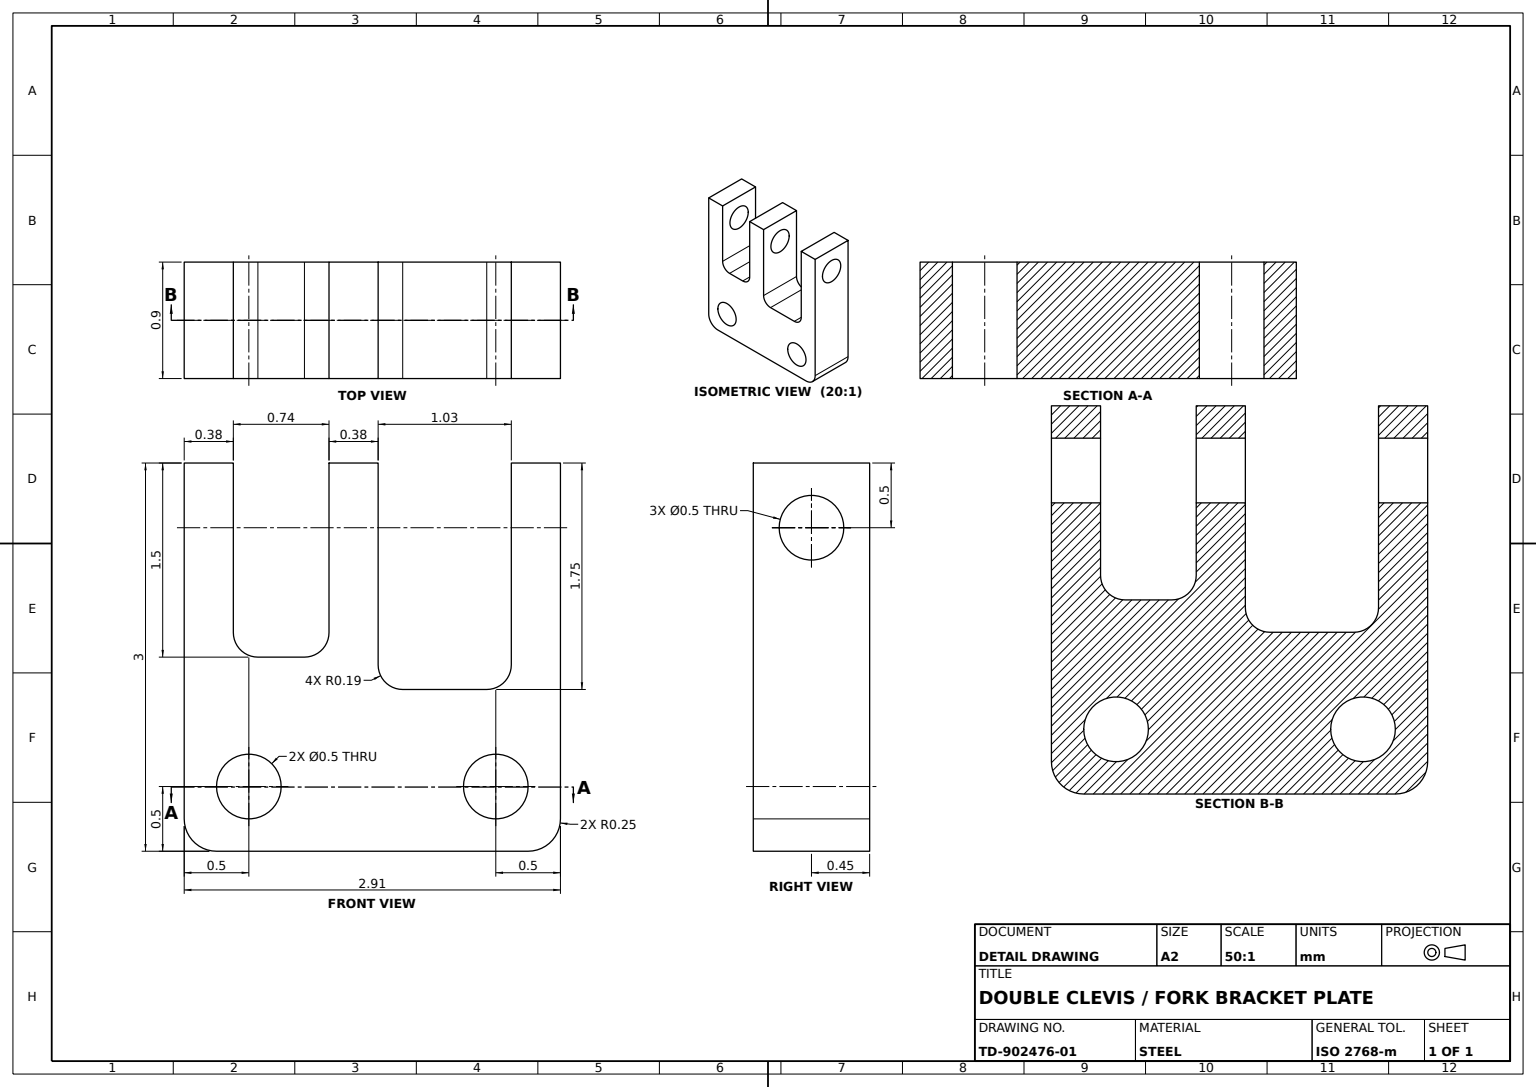
from build123d import *

# Parameters (mm, degrees)
BRACKET_PLATE_PROFILE_W = 2.91
BRACKET_PLATE_PROFILE_H = 0.9
BRACKET_PLATE_DEPTH     = 3
CORNER_FILLET_R0_25_R   = 0.25
PRONG_SLOTS_DEPTH       = 3
MOUNTING_HOLES_SKETCH_R = 0.25
MOUNTING_HOLES_2X_DEPTH = 3
CROSS_PIN_BORE_SKETCH_R = 0.25
CROSS_PIN_BORE_DEPTH    = 5.203641279


with BuildPart() as part:
    # Bracket Plate Profile → Bracket Plate (new body)
    with BuildSketch(Plane(origin=(0, 0, 0), x_dir=(1, 0, 0), z_dir=(0, 1, 0))):
        Rectangle(BRACKET_PLATE_PROFILE_W, BRACKET_PLATE_PROFILE_H)
    extrude(amount=BRACKET_PLATE_DEPTH)

    # Corner Fillet R0.25
    corner_fillet_r0_25_edges = [part.edges().sort_by_distance(p)[0] for p in [
        (-1.455, 0, 0),
        (1.455, 0, 0),
    ]]
    fillet(corner_fillet_r0_25_edges, radius=CORNER_FILLET_R0_25_R)

    # Prong Slots Sketch → Prong Slots (cut)
    with BuildSketch(Plane.XY.offset(0.45)):
        with BuildLine():
            Line((-1.075, 3), (-1.075, 1.69))
            ThreePointArc((-1.075, 1.69), (-1.019350288, 1.555649712), (-0.885, 1.5))
            Line((-0.885, 1.5), (-0.525, 1.5))
            ThreePointArc((-0.525, 1.5), (-0.390649712, 1.555649712), (-0.335, 1.69))
            Line((-0.335, 1.69), (-0.335, 3))
            Line((-0.335, 3), (-1.075, 3))
        make_face()
        with BuildLine():
            Line((1.075, 3), (1.075, 1.44))
            ThreePointArc((1.075, 1.44), (1.019350288, 1.305649712), (0.885, 1.25))
            Line((0.885, 1.25), (0.235, 1.25))
            ThreePointArc((0.235, 1.25), (0.100649712, 1.305649712), (0.045, 1.44))
            Line((0.045, 1.44), (0.045, 3))
            Line((0.045, 3), (1.075, 3))
        make_face()
    extrude(amount=-PRONG_SLOTS_DEPTH, mode=Mode.SUBTRACT)

    # Mounting Holes Sketch → Mounting Holes 2x (cut)
    with BuildSketch(Plane.XY.offset(0.45)):
        with Locations((-0.955, 0.5)):
            Circle(MOUNTING_HOLES_SKETCH_R)
        with Locations((0.955, 0.5)):
            Circle(MOUNTING_HOLES_SKETCH_R)
    extrude(amount=-MOUNTING_HOLES_2X_DEPTH, mode=Mode.SUBTRACT)

    # Cross Pin Bore Sketch → Cross Pin Bore (cut, through all)
    with BuildSketch(Plane(origin=(1.455, 0, 0), x_dir=(0, 0, -1), z_dir=(1, 0, 0))):
        with Locations((0, 2.5)):
            Circle(CROSS_PIN_BORE_SKETCH_R)
    extrude(amount=-CROSS_PIN_BORE_DEPTH, mode=Mode.SUBTRACT)


solid = part.part
